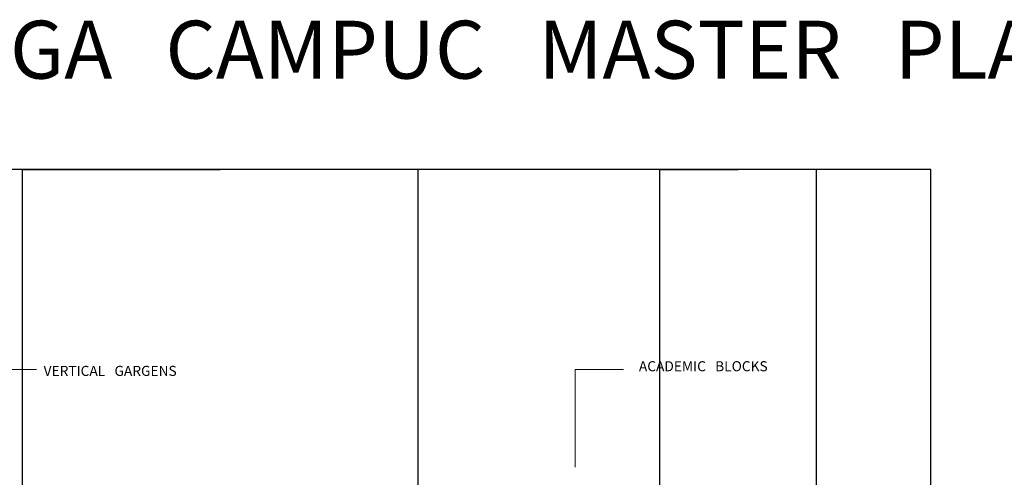
# Model space of a CAD drawing. Units: inches. Extents: x -32109 to 33221, y -19197 to 7608.
# Tile 23 of 25: x 6939 to 19011, y 1998 to 7608. Entities that reach past the tile are written whole.
import ezdxf

# ---------------------------------------------------------------- set-up
doc = ezdxf.new("R2010")
doc.units = ezdxf.units.IN
doc.header["$MEASUREMENT"] = 0
for name, color, linetype, lineweight in [('A-ANNO-DIMS', 2, 'Continuous', 18), ('A-ANNO-NOTE', 2, 'Continuous', 18), ('A-ANNO-TEXT', 7, 'Continuous', 25)]:
    doc.layers.add(name, color=color, linetype=linetype, lineweight=lineweight)
doc.styles.get("Standard").update_dxf_attribs({"font": 'arial.ttf'})
doc.dimstyles.get("Standard").update_dxf_attribs({"dimtxt": 0.18, "dimasz": 0.18, "dimexe": 0.18, "dimexo": 0.0625, "dimgap": 0.09, "dimtad": 0, "dimtih": 1, "dimtoh": 1, "dimdec": 4, "dimzin": 0, "dimdsep": 46, "dimtxsty": 'Standard', "dimcen": 0.09, "dimadec": 0, "dimazin": 0, "dimtfac": 1, "dimtdec": 4, "dimtofl": 0, "dimtmove": 0, "dimatfit": 3, "dimfxl": 1, "dimtolj": 1, "dimtzin": 0, "dimarcsym": 0})

# ---------------------------------------------------------------- blocks, each defined once
blk = doc.blocks.new('*D10')
at = {"layer": 'A-ANNO-DIMS', "color": 0, "lineweight": -2, "transparency": 16777216}
for p, q in [((-18512.646816, -110.179138), (-18512.646816, 5772.015489000001)), ((-18512.466816, 5771.835489), (-202.0927503703958, 5771.835489)), ((18109.136745, 5771.835489), (-201.2373206296045, 5771.835489)), ((18109.316745, -101.537382), (18109.316745, 5772.015489000001))]:
    blk.add_line(p, q, dxfattribs=at)
at = {"layer": 'A-ANNO-DIMS', "color": 0, "transparency": 16777216}
for points in [[(-18512.466816, 5771.865488999999), (-18512.466816, 5771.805489000001), (-18512.646816, 5771.835489)], [(18109.136745, 5771.865488999999), (18109.136745, 5771.805489000001), (18109.316745, 5771.835489)]]:
    blk.add_solid(points, dxfattribs=at)
at = {"layer": 'Defpoints', "color": 0, "transparency": 16777216}
for p in [(18109.316745, 5771.835489), (-18512.646816, -110.241638), (18109.316745, -101.599882)]:
    blk.add_point(p, dxfattribs=at)
at = {"layer": 'A-ANNO-DIMS', "color": 0, "transparency": 16777216, "insert": (-201.6650355000002, 5771.835489), "char_height": 0.18, "attachment_point": 5}
blk.add_mtext('\\A1;36622', dxfattribs=at)
blk = doc.blocks.new('*D66')
at = {"layer": 'A-ANNO-DIMS', "color": 0, "lineweight": -2, "transparency": 16777216}
for p, q in [((14786.395525, 963.792278), (14786.395525, 5772.015489000001)), ((14786.575525, 5771.835489), (15747.65543045975, 5771.835489)), ((16709.644913, 5771.835489), (15748.56500754024, 5771.835489)), ((16709.824913, 963.792278), (16709.824913, 5772.015489000001))]:
    blk.add_line(p, q, dxfattribs=at)
at = {"layer": 'A-ANNO-DIMS', "color": 0, "transparency": 16777216}
for points in [[(14786.575525, 5771.865488999999), (14786.575525, 5771.805489000001), (14786.395525, 5771.835489)], [(16709.644913, 5771.865488999999), (16709.644913, 5771.805489000001), (16709.824913, 5771.835489)]]:
    blk.add_solid(points, dxfattribs=at)
at = {"layer": 'Defpoints', "color": 0, "transparency": 16777216}
for p in [(16709.824913, 5771.835489), (14786.395525, 963.729778), (16709.824913, 963.729778)]:
    blk.add_point(p, dxfattribs=at)
at = {"layer": 'A-ANNO-DIMS', "color": 0, "transparency": 16777216, "insert": (15748.110219, 5771.835489), "char_height": 0.18, "attachment_point": 5}
blk.add_mtext('\\A1;1923.4', dxfattribs=at)
blk = doc.blocks.new('*D73')
at = {"layer": 'A-ANNO-DIMS', "color": 0, "lineweight": -2, "transparency": 16777216}
for p, q in [((6972.547547000001, 772.890849), (6972.547547000001, 5772.015489000001)), ((6972.727547000001, 5771.835489), (9397.548274536153, 5771.835489)), ((11823.059043, 5771.835489), (9398.238315463848, 5771.835489)), ((11823.239043, 772.890849), (11823.239043, 5772.015489000001))]:
    blk.add_line(p, q, dxfattribs=at)
at = {"layer": 'A-ANNO-DIMS', "color": 0, "transparency": 16777216}
for points in [[(6972.727547000001, 5771.865488999999), (6972.727547000001, 5771.805489000001), (6972.547547000001, 5771.835489)], [(11823.059043, 5771.865488999999), (11823.059043, 5771.805489000001), (11823.239043, 5771.835489)]]:
    blk.add_solid(points, dxfattribs=at)
at = {"layer": 'Defpoints', "color": 0, "transparency": 16777216}
for p in [(11823.239043, 5771.835489), (6972.547547000001, 772.8283489999999), (11823.239043, 772.8283489999999)]:
    blk.add_point(p, dxfattribs=at)
at = {"layer": 'A-ANNO-DIMS', "color": 0, "transparency": 16777216, "insert": (9397.893295000002, 5771.835489), "char_height": 0.18, "attachment_point": 5}
blk.add_mtext('\\A1;4851', dxfattribs=at)

msp = doc.modelspace()

# ---------------------------------------------------------------- linework, layer by layer
at = {"layer": 'A-ANNO-NOTE'}
for p, q in [((6402.717398849883, 3321.835488633435), (7145.280624769163, 3321.835488633435)), ((13748.90576412412, 2121.956467826327), (13748.90576412412, 3321.835488633435)), ((13748.90576412412, 3321.835488633435), (14342.95619528868, 3321.835488633435))]:
    msp.add_line(p, q, dxfattribs=at)

# ---------------------------------------------------------------- texts
at = {"layer": 'A-ANNO-TEXT'}
for s, height, p in [('COMPREHENSIVE   ARCHITECTURAL   INTERLOCKING    CUBE   MEGA   CAMPUC   MASTER   PLAN ', 709.7949465747753, (-22238.10681632875, 6885.298304043546)), ('ACADEMIC   BLOCKS', 123.5547426012344, (14530.84773739427, 3298.097887211458)), ('VERTICAL   GARGENS ', 123.5547426012344, (7232.388977008639, 3241.133260178532))]:
    msp.add_text(s, height=height, dxfattribs=at).set_placement(p)

# ---------------------------------------------------------------- dimensions: what is measured, and where the dimension line sits
at = {"layer": 'A-ANNO-DIMS'}
for base, p1, p2, override, picture, middle in [((18109.316745, 5771.835489), (-18512.646816, -110.241638), (18109.316745, -101.599882), {"dimdec": 0, "dimlfac": 1, "dimrnd": 0, "dimzin": 0, "dimdsep": 46, "dimlunit": 2}, '*D10', (-201.6650355000002, 5771.835489)), ((11823.239043, 5771.835489), (6972.547547000001, 772.8283489999999), (11823.239043, 772.8283489999999), {"dimdec": 0, "dimlfac": 1, "dimrnd": 0, "dimzin": 0, "dimdsep": 46, "dimlunit": 2}, '*D73', (9397.893295000002, 5771.835489)), ((16709.824913, 5771.835489), (14786.395525, 963.729778), (16709.824913, 963.729778), {"dimdec": 1, "dimlfac": 1, "dimrnd": 0, "dimzin": 0, "dimdsep": 46, "dimlunit": 2}, '*D66', (15748.110219, 5771.835489))]:
    dim = msp.add_linear_dim(base=base, p1=p1, p2=p2, dimstyle='Standard', override=override, dxfattribs=at)
    dim.commit()
    dim.dimension.update_dxf_attribs({"geometry": picture, "text_midpoint": middle})

doc.saveas('drawing.dxf')
